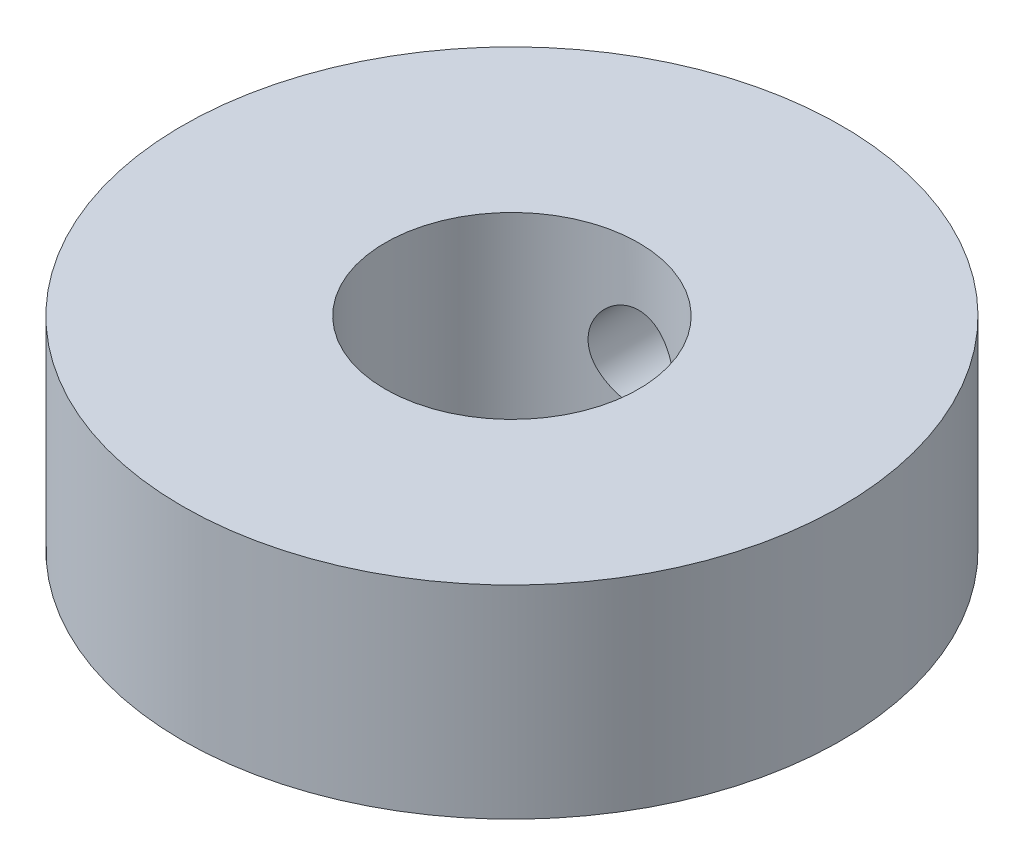
from build123d import *

# Parameters (mm, degrees)
RING_PROFILE_13_X_5_R   = 6.5
RING_PROFILE_13_X_5_R_2 = 2.5
COVER_RING_DEPTH        = 4
RADIAL_HOLE_PROFILE_2_R = 0.85
RADIAL_HOLE_2_DEPTH     = 7


with BuildPart() as part:
    # Ring Profile Ø13 x Ø5 → Cover Ring (new body)
    with BuildSketch(Plane(origin=(0, 0, 0), x_dir=(1, 0, 0), z_dir=(0, 1, 0))):
        with Locations(Location((0, 0, 0), (0, 0, 270))):
            Circle(RING_PROFILE_13_X_5_R)
        with Locations(Location((0, 0, 0), (0, 0, 270))):
            Circle(RING_PROFILE_13_X_5_R_2, mode=Mode.SUBTRACT)
    extrude(amount=COVER_RING_DEPTH)

    # Radial Hole Profile Ø2 → Radial Hole Ø2 (cut)
    with BuildSketch(Plane.XY):
        with Locations(Location((0, 2, 0), (0, 0, 90))):
            Circle(RADIAL_HOLE_PROFILE_2_R)
    extrude(amount=-RADIAL_HOLE_2_DEPTH, mode=Mode.SUBTRACT)


solid = part.part
